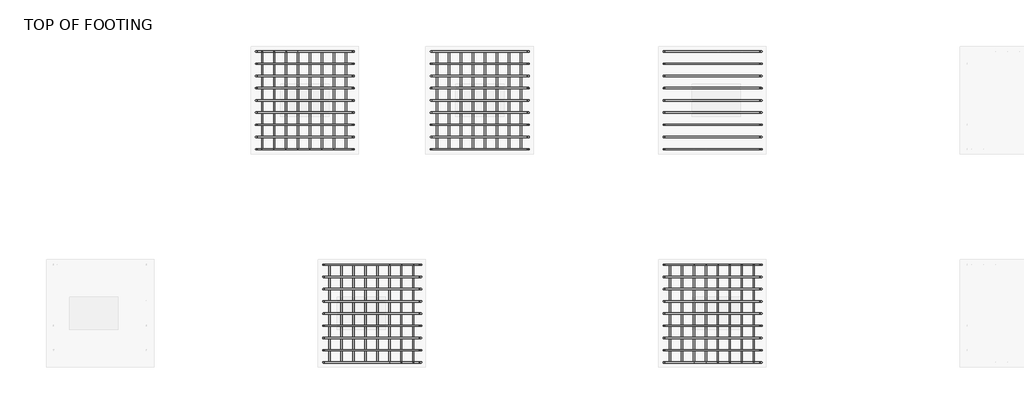
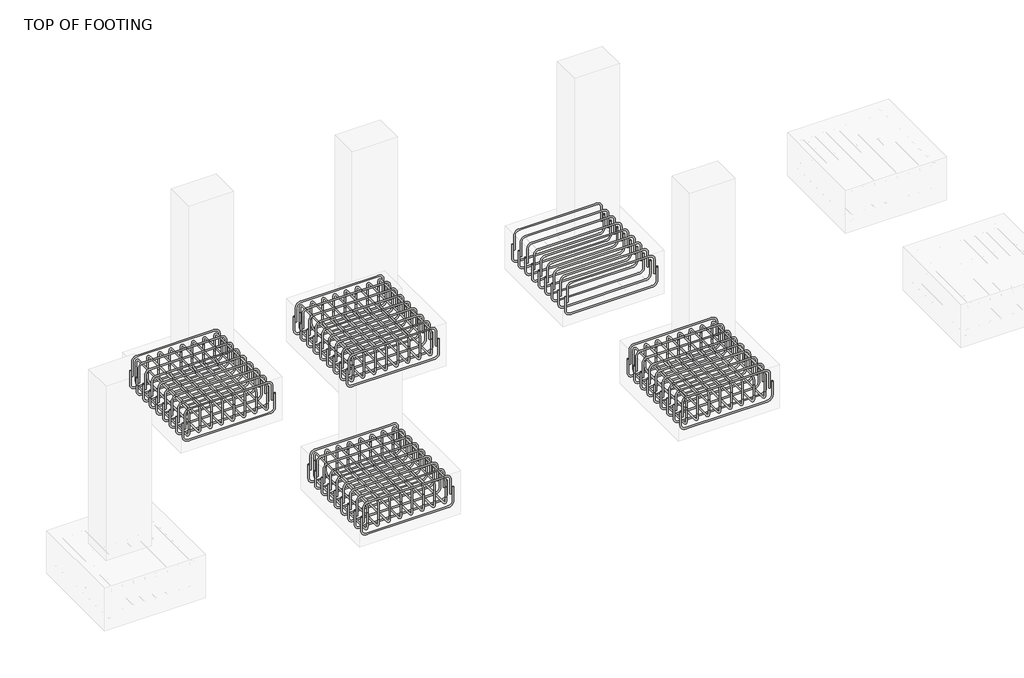
# One storey, part 17 of 20: 18 reinforcing bars.
"""IFC4 building model written with IfcOpenShell, lengths in millimetres."""

from ifc_helpers import new_model, si_unit, point, frame, origin, place, context, project, spatial, polyline, circle_curve, trimmed, segment, composite_curve, source, transform, mapped, element, save
from ifc_brep_helpers import swept_disk

model = new_model("IFC4")

# Units and contexts
model_context = context("Model", 3, world=origin())
ifc_project = project(units=[si_unit("LENGTHUNIT", "METRE", prefix="MILLI")], contexts=[model_context])

# Site, building, storey
site = spatial("IfcSite", under=ifc_project)
building = spatial("IfcBuilding", under=site)
storey = spatial("IfcBuildingStorey", under=building, Name="TOP OF FOOTING", Elevation=-1828.8)

# Reinforcing bars
placement = place(None, origin())
reinforcing_bar_shape = source(origin(), model_context, "Body", "SolidModel", [
    swept_disk(composite_curve([segment(polyline([(6636.1748054, 14441.1679708, -2006.6587682), (6636.1748054, 14441.1679708, -2153.9587682)]), True, "CONTINUOUS"), segment(trimmed(circle_curve(frame((6589.8248054, 14441.1679708, -2153.9587682), z_axis=(0.0, 1.0, 0.0), x_axis=(46.350000000000364, 0.0, 0.0)), 46.35), [point((6636.1748054, 14441.1679708, -2153.9587682))], [point((6589.8248054, 14441.1679708, -2200.3087682))], True, "CARTESIAN"), True, "CONTINUOUS"), segment(polyline([(6589.8248054, 14441.1679708, -2200.3087682), (5775.2248054, 14441.1679708, -2200.3087682)]), True, "CONTINUOUS"), segment(trimmed(circle_curve(frame((5775.2248054, 14441.1679708, -2153.9587682), z_axis=(0.0, 1.0, 0.0), x_axis=(0.0, 0.0, -46.34999999999991)), 46.35), [point((5775.2248054, 14441.1679708, -2200.3087682))], [point((5728.8748054, 14441.1679708, -2153.9587682))], True, "CARTESIAN"), True, "CONTINUOUS"), segment(polyline([(5728.8748054, 14441.1679708, -2153.9587682), (5728.8748054, 14441.1679708, -2006.6587682)]), True, "CONTINUOUS")], self_intersect=False), 6.35),
])
element("IfcReinforcingBar", 1, at=placement, inside=storey, context=model_context, shape_type="MappedRepresentation", body=[
    mapped(reinforcing_bar_shape, transform((0.0, 0.0, 0.0), x_axis=(1.0, 0.0, 0.0), y_axis=(0.0, 1.0, 0.0), z_axis=(0.0, 0.0, 1.0))),
    mapped(reinforcing_bar_shape, transform((0.0, -113.4125, 0.0), x_axis=(1.0, 0.0, 0.0), y_axis=(0.0, 1.0, 0.0), z_axis=(0.0, 0.0, 1.0))),
    mapped(reinforcing_bar_shape, transform((0.0, -226.825, 0.0), x_axis=(1.0, 0.0, 0.0), y_axis=(0.0, 1.0, 0.0), z_axis=(0.0, 0.0, 1.0))),
    mapped(reinforcing_bar_shape, transform((0.0, -340.2375, 0.0), x_axis=(1.0, 0.0, 0.0), y_axis=(0.0, 1.0, 0.0), z_axis=(0.0, 0.0, 1.0))),
    mapped(reinforcing_bar_shape, transform((0.0, -453.65, 0.0), x_axis=(1.0, 0.0, 0.0), y_axis=(0.0, 1.0, 0.0), z_axis=(0.0, 0.0, 1.0))),
    mapped(reinforcing_bar_shape, transform((0.0, -567.0625, 0.0), x_axis=(1.0, 0.0, 0.0), y_axis=(0.0, 1.0, 0.0), z_axis=(0.0, 0.0, 1.0))),
    mapped(reinforcing_bar_shape, transform((0.0, -680.475, 0.0), x_axis=(1.0, 0.0, 0.0), y_axis=(0.0, 1.0, 0.0), z_axis=(0.0, 0.0, 1.0))),
    mapped(reinforcing_bar_shape, transform((0.0, -793.8875, 0.0), x_axis=(1.0, 0.0, 0.0), y_axis=(0.0, 1.0, 0.0), z_axis=(0.0, 0.0, 1.0))),
    mapped(reinforcing_bar_shape, transform((0.0, -907.3, 0.0), x_axis=(1.0, 0.0, 0.0), y_axis=(0.0, 1.0, 0.0), z_axis=(0.0, 0.0, 1.0))),
])
reinforcing_bar_2_shape = source(origin(), model_context, "Body", "SolidModel", [
    swept_disk(composite_curve([segment(polyline([(5748.3489167, 14441.1679708, -2068.8), (5748.3489167, 14441.1679708, -1921.5)]), True, "CONTINUOUS"), segment(trimmed(circle_curve(frame((5794.6989167, 14441.1679708, -1921.5), z_axis=(0.0, 1.0, 0.0), x_axis=(-46.350000000000364, 0.0, 0.0)), 46.35), [point((5748.3489167, 14441.1679708, -1921.5))], [point((5794.6989167, 14441.1679708, -1875.15))], True, "CARTESIAN"), True, "CONTINUOUS"), segment(polyline([(5794.6989167, 14441.1679708, -1875.15), (6564.1623164, 14441.1679708, -1875.15)]), True, "CONTINUOUS"), segment(trimmed(circle_curve(frame((6564.1623164, 14441.1679708, -1921.5), z_axis=(0.0, 1.0, 0.0), x_axis=(0.0, 0.0, 46.34999999999991)), 46.35), [point((6564.1623164, 14441.1679708, -1875.15))], [point((6610.5123164, 14441.1679708, -1921.5))], True, "CARTESIAN"), True, "CONTINUOUS"), segment(polyline([(6610.5123164, 14441.1679708, -1921.5), (6610.5123164, 14441.1679708, -2068.8)]), True, "CONTINUOUS")], self_intersect=False), 6.35),
])
element("IfcReinforcingBar", 2, at=placement, inside=storey, context=model_context, shape_type="MappedRepresentation", body=[
    mapped(reinforcing_bar_2_shape, transform((0.0, 0.0, 0.0), x_axis=(1.0, 0.0, 0.0), y_axis=(0.0, 1.0, 0.0), z_axis=(0.0, 0.0, 1.0))),
    mapped(reinforcing_bar_2_shape, transform((0.0, -113.4125, 0.0), x_axis=(1.0, 0.0, 0.0), y_axis=(0.0, 1.0, 0.0), z_axis=(0.0, 0.0, 1.0))),
    mapped(reinforcing_bar_2_shape, transform((0.0, -226.825, 0.0), x_axis=(1.0, 0.0, 0.0), y_axis=(0.0, 1.0, 0.0), z_axis=(0.0, 0.0, 1.0))),
    mapped(reinforcing_bar_2_shape, transform((0.0, -340.2375, 0.0), x_axis=(1.0, 0.0, 0.0), y_axis=(0.0, 1.0, 0.0), z_axis=(0.0, 0.0, 1.0))),
    mapped(reinforcing_bar_2_shape, transform((0.0, -453.65, 0.0), x_axis=(1.0, 0.0, 0.0), y_axis=(0.0, 1.0, 0.0), z_axis=(0.0, 0.0, 1.0))),
    mapped(reinforcing_bar_2_shape, transform((0.0, -567.0625, 0.0), x_axis=(1.0, 0.0, 0.0), y_axis=(0.0, 1.0, 0.0), z_axis=(0.0, 0.0, 1.0))),
    mapped(reinforcing_bar_2_shape, transform((0.0, -680.475, 0.0), x_axis=(1.0, 0.0, 0.0), y_axis=(0.0, 1.0, 0.0), z_axis=(0.0, 0.0, 1.0))),
    mapped(reinforcing_bar_2_shape, transform((0.0, -793.8875, 0.0), x_axis=(1.0, 0.0, 0.0), y_axis=(0.0, 1.0, 0.0), z_axis=(0.0, 0.0, 1.0))),
    mapped(reinforcing_bar_2_shape, transform((0.0, -907.3, 0.0), x_axis=(1.0, 0.0, 0.0), y_axis=(0.0, 1.0, 0.0), z_axis=(0.0, 0.0, 1.0))),
])
reinforcing_bar_3_shape = source(origin(), model_context, "Body", "SolidModel", [
    swept_disk(composite_curve([segment(polyline([(6564.677844, 14441.1679708, -2086.1951968), (6564.677844, 14441.1679708, -1938.8951968)]), True, "CONTINUOUS"), segment(trimmed(circle_curve(frame((6564.677844, 14394.8179708, -1938.8951968), z_axis=(1.0, 0.0, 0.0), x_axis=(0.0, 46.349999999998545, 0.0)), 46.35), [point((6564.677844, 14441.1679708, -1938.8951968))], [point((6564.677844, 14394.8179708, -1892.5451968))], True, "CARTESIAN"), True, "CONTINUOUS"), segment(polyline([(6564.677844, 14394.8179708, -1892.5451968), (6564.677844, 13580.2179708, -1892.5451968)]), True, "CONTINUOUS"), segment(trimmed(circle_curve(frame((6564.677844, 13580.2179708, -1938.8951968), z_axis=(1.0, 0.0, 0.0), x_axis=(0.0, 0.0, 46.34999999999991)), 46.35), [point((6564.677844, 13580.2179708, -1892.5451968))], [point((6564.677844, 13533.8679708, -1938.8951968))], True, "CARTESIAN"), True, "CONTINUOUS"), segment(polyline([(6564.677844, 13533.8679708, -1938.8951968), (6564.677844, 13533.8679708, -2086.1951968)]), True, "CONTINUOUS")], self_intersect=False), 6.35),
])
element("IfcReinforcingBar", 3, at=placement, inside=storey, context=model_context, shape_type="MappedRepresentation", body=[
    mapped(reinforcing_bar_3_shape, transform((0.0, 0.0, 0.0), x_axis=(1.0, 0.0, 0.0), y_axis=(0.0, 1.0, 0.0), z_axis=(0.0, 0.0, 1.0))),
    mapped(reinforcing_bar_3_shape, transform((-111.2862402, 0.0, 0.0), x_axis=(1.0, 0.0, 0.0), y_axis=(0.0, 1.0, 0.0), z_axis=(0.0, 0.0, 1.0))),
    mapped(reinforcing_bar_3_shape, transform((-222.5724804, 0.0, 0.0), x_axis=(1.0, 0.0, 0.0), y_axis=(0.0, 1.0, 0.0), z_axis=(0.0, 0.0, 1.0))),
    mapped(reinforcing_bar_3_shape, transform((-333.8587205, 0.0, 0.0), x_axis=(1.0, 0.0, 0.0), y_axis=(0.0, 1.0, 0.0), z_axis=(0.0, 0.0, 1.0))),
    mapped(reinforcing_bar_3_shape, transform((-445.1449607, 0.0, 0.0), x_axis=(1.0, 0.0, 0.0), y_axis=(0.0, 1.0, 0.0), z_axis=(0.0, 0.0, 1.0))),
    mapped(reinforcing_bar_3_shape, transform((-556.4312009, 0.0, 0.0), x_axis=(1.0, 0.0, 0.0), y_axis=(0.0, 1.0, 0.0), z_axis=(0.0, 0.0, 1.0))),
    mapped(reinforcing_bar_3_shape, transform((-667.7174411, 0.0, 0.0), x_axis=(1.0, 0.0, 0.0), y_axis=(0.0, 1.0, 0.0), z_axis=(0.0, 0.0, 1.0))),
    mapped(reinforcing_bar_3_shape, transform((-779.0036813, 0.0, 0.0), x_axis=(1.0, 0.0, 0.0), y_axis=(0.0, 1.0, 0.0), z_axis=(0.0, 0.0, 1.0))),
])
reinforcing_bar_4_shape = source(origin(), model_context, "Body", "SolidModel", [
    swept_disk(composite_curve([segment(polyline([(5785.6741627, 14441.1679708, -1979.1645013), (5785.6741627, 14441.1679708, -2126.4645013)]), True, "CONTINUOUS"), segment(trimmed(circle_curve(frame((5785.6741627, 14394.8179708, -2126.4645013), z_axis=(-1.0, 0.0, 0.0), x_axis=(0.0, 46.349999999998545, 0.0)), 46.35), [point((5785.6741627, 14441.1679708, -2126.4645013))], [point((5785.6741627, 14394.8179708, -2172.8145013))], True, "CARTESIAN"), True, "CONTINUOUS"), segment(polyline([(5785.6741627, 14394.8179708, -2172.8145013), (5785.6741627, 13580.2179708, -2172.8145013)]), True, "CONTINUOUS"), segment(trimmed(circle_curve(frame((5785.6741627, 13580.2179708, -2126.4645013), z_axis=(-1.0, 0.0, 0.0), x_axis=(0.0, 0.0, -46.34999999999991)), 46.35), [point((5785.6741627, 13580.2179708, -2172.8145013))], [point((5785.6741627, 13533.8679708, -2126.4645013))], True, "CARTESIAN"), True, "CONTINUOUS"), segment(polyline([(5785.6741627, 13533.8679708, -2126.4645013), (5785.6741627, 13533.8679708, -1979.1645013)]), True, "CONTINUOUS")], self_intersect=False), 6.35),
])
element("IfcReinforcingBar", 4, at=placement, inside=storey, context=model_context, shape_type="MappedRepresentation", body=[
    mapped(reinforcing_bar_4_shape, transform((0.0, 0.0, 0.0), x_axis=(1.0, 0.0, 0.0), y_axis=(0.0, 1.0, 0.0), z_axis=(0.0, 0.0, 1.0))),
    mapped(reinforcing_bar_4_shape, transform((111.2862402, 0.0, 0.0), x_axis=(1.0, 0.0, 0.0), y_axis=(0.0, 1.0, 0.0), z_axis=(0.0, 0.0, 1.0))),
    mapped(reinforcing_bar_4_shape, transform((222.5724804, 0.0, 0.0), x_axis=(1.0, 0.0, 0.0), y_axis=(0.0, 1.0, 0.0), z_axis=(0.0, 0.0, 1.0))),
    mapped(reinforcing_bar_4_shape, transform((333.8587205, 0.0, 0.0), x_axis=(1.0, 0.0, 0.0), y_axis=(0.0, 1.0, 0.0), z_axis=(0.0, 0.0, 1.0))),
    mapped(reinforcing_bar_4_shape, transform((445.1449607, 0.0, 0.0), x_axis=(1.0, 0.0, 0.0), y_axis=(0.0, 1.0, 0.0), z_axis=(0.0, 0.0, 1.0))),
    mapped(reinforcing_bar_4_shape, transform((556.4312009, 0.0, 0.0), x_axis=(1.0, 0.0, 0.0), y_axis=(0.0, 1.0, 0.0), z_axis=(0.0, 0.0, 1.0))),
    mapped(reinforcing_bar_4_shape, transform((667.7174411, 0.0, 0.0), x_axis=(1.0, 0.0, 0.0), y_axis=(0.0, 1.0, 0.0), z_axis=(0.0, 0.0, 1.0))),
    mapped(reinforcing_bar_4_shape, transform((779.0036813, 0.0, 0.0), x_axis=(1.0, 0.0, 0.0), y_axis=(0.0, 1.0, 0.0), z_axis=(0.0, 0.0, 1.0))),
])
reinforcing_bar_5_shape = source(origin(), model_context, "Body", "SolidModel", [
    swept_disk(composite_curve([segment(polyline([(8260.5179014, 14441.1679708, -2006.6587682), (8260.5179014, 14441.1679708, -2153.9587682)]), True, "CONTINUOUS"), segment(trimmed(circle_curve(frame((8214.1679014, 14441.1679708, -2153.9587682), z_axis=(0.0, 1.0, 0.0), x_axis=(46.350000000000364, 0.0, 0.0)), 46.35), [point((8260.5179014, 14441.1679708, -2153.9587682))], [point((8214.1679014, 14441.1679708, -2200.3087682))], True, "CARTESIAN"), True, "CONTINUOUS"), segment(polyline([(8214.1679014, 14441.1679708, -2200.3087682), (7399.5679014, 14441.1679708, -2200.3087682)]), True, "CONTINUOUS"), segment(trimmed(circle_curve(frame((7399.5679014, 14441.1679708, -2153.9587682), z_axis=(0.0, 1.0, 0.0), x_axis=(0.0, 0.0, -46.34999999999991)), 46.35), [point((7399.5679014, 14441.1679708, -2200.3087682))], [point((7353.2179014, 14441.1679708, -2153.9587682))], True, "CARTESIAN"), True, "CONTINUOUS"), segment(polyline([(7353.2179014, 14441.1679708, -2153.9587682), (7353.2179014, 14441.1679708, -2006.6587682)]), True, "CONTINUOUS")], self_intersect=False), 6.35),
])
element("IfcReinforcingBar", 5, at=placement, inside=storey, context=model_context, shape_type="MappedRepresentation", body=[
    mapped(reinforcing_bar_5_shape, transform((0.0, 0.0, 0.0), x_axis=(1.0, 0.0, 0.0), y_axis=(0.0, 1.0, 0.0), z_axis=(0.0, 0.0, 1.0))),
    mapped(reinforcing_bar_5_shape, transform((0.0, -113.4125, 0.0), x_axis=(1.0, 0.0, 0.0), y_axis=(0.0, 1.0, 0.0), z_axis=(0.0, 0.0, 1.0))),
    mapped(reinforcing_bar_5_shape, transform((0.0, -226.825, 0.0), x_axis=(1.0, 0.0, 0.0), y_axis=(0.0, 1.0, 0.0), z_axis=(0.0, 0.0, 1.0))),
    mapped(reinforcing_bar_5_shape, transform((0.0, -340.2375, 0.0), x_axis=(1.0, 0.0, 0.0), y_axis=(0.0, 1.0, 0.0), z_axis=(0.0, 0.0, 1.0))),
    mapped(reinforcing_bar_5_shape, transform((0.0, -453.65, 0.0), x_axis=(1.0, 0.0, 0.0), y_axis=(0.0, 1.0, 0.0), z_axis=(0.0, 0.0, 1.0))),
    mapped(reinforcing_bar_5_shape, transform((0.0, -567.0625, 0.0), x_axis=(1.0, 0.0, 0.0), y_axis=(0.0, 1.0, 0.0), z_axis=(0.0, 0.0, 1.0))),
    mapped(reinforcing_bar_5_shape, transform((0.0, -680.475, 0.0), x_axis=(1.0, 0.0, 0.0), y_axis=(0.0, 1.0, 0.0), z_axis=(0.0, 0.0, 1.0))),
    mapped(reinforcing_bar_5_shape, transform((0.0, -793.8875, 0.0), x_axis=(1.0, 0.0, 0.0), y_axis=(0.0, 1.0, 0.0), z_axis=(0.0, 0.0, 1.0))),
    mapped(reinforcing_bar_5_shape, transform((0.0, -907.3, 0.0), x_axis=(1.0, 0.0, 0.0), y_axis=(0.0, 1.0, 0.0), z_axis=(0.0, 0.0, 1.0))),
])
reinforcing_bar_6_shape = source(origin(), model_context, "Body", "SolidModel", [
    swept_disk(composite_curve([segment(polyline([(7372.6920127, 14441.1679708, -2068.8), (7372.6920127, 14441.1679708, -1921.5)]), True, "CONTINUOUS"), segment(trimmed(circle_curve(frame((7419.0420127, 14441.1679708, -1921.5), z_axis=(0.0, 1.0, 0.0), x_axis=(-46.349999999999454, 0.0, 0.0)), 46.35), [point((7372.6920127, 14441.1679708, -1921.5))], [point((7419.0420127, 14441.1679708, -1875.15))], True, "CARTESIAN"), True, "CONTINUOUS"), segment(polyline([(7419.0420127, 14441.1679708, -1875.15), (8188.5054124, 14441.1679708, -1875.15)]), True, "CONTINUOUS"), segment(trimmed(circle_curve(frame((8188.5054124, 14441.1679708, -1921.5), z_axis=(0.0, 1.0, 0.0), x_axis=(0.0, 0.0, 46.34999999999991)), 46.35), [point((8188.5054124, 14441.1679708, -1875.15))], [point((8234.8554124, 14441.1679708, -1921.5))], True, "CARTESIAN"), True, "CONTINUOUS"), segment(polyline([(8234.8554124, 14441.1679708, -1921.5), (8234.8554124, 14441.1679708, -2068.8)]), True, "CONTINUOUS")], self_intersect=False), 6.35),
])
element("IfcReinforcingBar", 6, at=placement, inside=storey, context=model_context, shape_type="MappedRepresentation", body=[
    mapped(reinforcing_bar_6_shape, transform((0.0, 0.0, 0.0), x_axis=(1.0, 0.0, 0.0), y_axis=(0.0, 1.0, 0.0), z_axis=(0.0, 0.0, 1.0))),
    mapped(reinforcing_bar_6_shape, transform((0.0, -113.4125, 0.0), x_axis=(1.0, 0.0, 0.0), y_axis=(0.0, 1.0, 0.0), z_axis=(0.0, 0.0, 1.0))),
    mapped(reinforcing_bar_6_shape, transform((0.0, -226.825, 0.0), x_axis=(1.0, 0.0, 0.0), y_axis=(0.0, 1.0, 0.0), z_axis=(0.0, 0.0, 1.0))),
    mapped(reinforcing_bar_6_shape, transform((0.0, -340.2375, 0.0), x_axis=(1.0, 0.0, 0.0), y_axis=(0.0, 1.0, 0.0), z_axis=(0.0, 0.0, 1.0))),
    mapped(reinforcing_bar_6_shape, transform((0.0, -453.65, 0.0), x_axis=(1.0, 0.0, 0.0), y_axis=(0.0, 1.0, 0.0), z_axis=(0.0, 0.0, 1.0))),
    mapped(reinforcing_bar_6_shape, transform((0.0, -567.0625, 0.0), x_axis=(1.0, 0.0, 0.0), y_axis=(0.0, 1.0, 0.0), z_axis=(0.0, 0.0, 1.0))),
    mapped(reinforcing_bar_6_shape, transform((0.0, -680.475, 0.0), x_axis=(1.0, 0.0, 0.0), y_axis=(0.0, 1.0, 0.0), z_axis=(0.0, 0.0, 1.0))),
    mapped(reinforcing_bar_6_shape, transform((0.0, -793.8875, 0.0), x_axis=(1.0, 0.0, 0.0), y_axis=(0.0, 1.0, 0.0), z_axis=(0.0, 0.0, 1.0))),
    mapped(reinforcing_bar_6_shape, transform((0.0, -907.3, 0.0), x_axis=(1.0, 0.0, 0.0), y_axis=(0.0, 1.0, 0.0), z_axis=(0.0, 0.0, 1.0))),
])
reinforcing_bar_7_shape = source(origin(), model_context, "Body", "SolidModel", [
    swept_disk(composite_curve([segment(polyline([(8189.02094, 14441.1679708, -2086.1951968), (8189.02094, 14441.1679708, -1938.8951968)]), True, "CONTINUOUS"), segment(trimmed(circle_curve(frame((8189.02094, 14394.8179708, -1938.8951968), z_axis=(1.0, 0.0, 0.0), x_axis=(0.0, 46.349999999998545, 0.0)), 46.35), [point((8189.02094, 14441.1679708, -1938.8951968))], [point((8189.02094, 14394.8179708, -1892.5451968))], True, "CARTESIAN"), True, "CONTINUOUS"), segment(polyline([(8189.02094, 14394.8179708, -1892.5451968), (8189.02094, 13580.2179708, -1892.5451968)]), True, "CONTINUOUS"), segment(trimmed(circle_curve(frame((8189.02094, 13580.2179708, -1938.8951968), z_axis=(1.0, 0.0, 0.0), x_axis=(0.0, 0.0, 46.34999999999991)), 46.35), [point((8189.02094, 13580.2179708, -1892.5451968))], [point((8189.02094, 13533.8679708, -1938.8951968))], True, "CARTESIAN"), True, "CONTINUOUS"), segment(polyline([(8189.02094, 13533.8679708, -1938.8951968), (8189.02094, 13533.8679708, -2086.1951968)]), True, "CONTINUOUS")], self_intersect=False), 6.35),
])
element("IfcReinforcingBar", 7, at=placement, inside=storey, context=model_context, shape_type="MappedRepresentation", body=[
    mapped(reinforcing_bar_7_shape, transform((0.0, 0.0, 0.0), x_axis=(1.0, 0.0, 0.0), y_axis=(0.0, 1.0, 0.0), z_axis=(0.0, 0.0, 1.0))),
    mapped(reinforcing_bar_7_shape, transform((-111.2862402, 0.0, 0.0), x_axis=(1.0, 0.0, 0.0), y_axis=(0.0, 1.0, 0.0), z_axis=(0.0, 0.0, 1.0))),
    mapped(reinforcing_bar_7_shape, transform((-222.5724804, 0.0, 0.0), x_axis=(1.0, 0.0, 0.0), y_axis=(0.0, 1.0, 0.0), z_axis=(0.0, 0.0, 1.0))),
    mapped(reinforcing_bar_7_shape, transform((-333.8587205, 0.0, 0.0), x_axis=(1.0, 0.0, 0.0), y_axis=(0.0, 1.0, 0.0), z_axis=(0.0, 0.0, 1.0))),
    mapped(reinforcing_bar_7_shape, transform((-445.1449607, 0.0, 0.0), x_axis=(1.0, 0.0, 0.0), y_axis=(0.0, 1.0, 0.0), z_axis=(0.0, 0.0, 1.0))),
    mapped(reinforcing_bar_7_shape, transform((-556.4312009, 0.0, 0.0), x_axis=(1.0, 0.0, 0.0), y_axis=(0.0, 1.0, 0.0), z_axis=(0.0, 0.0, 1.0))),
    mapped(reinforcing_bar_7_shape, transform((-667.7174411, 0.0, 0.0), x_axis=(1.0, 0.0, 0.0), y_axis=(0.0, 1.0, 0.0), z_axis=(0.0, 0.0, 1.0))),
    mapped(reinforcing_bar_7_shape, transform((-779.0036813, 0.0, 0.0), x_axis=(1.0, 0.0, 0.0), y_axis=(0.0, 1.0, 0.0), z_axis=(0.0, 0.0, 1.0))),
])
reinforcing_bar_8_shape = source(origin(), model_context, "Body", "SolidModel", [
    swept_disk(composite_curve([segment(polyline([(7410.0172587, 14441.1679708, -1979.1645013), (7410.0172587, 14441.1679708, -2126.4645013)]), True, "CONTINUOUS"), segment(trimmed(circle_curve(frame((7410.0172587, 14394.8179708, -2126.4645013), z_axis=(-1.0, 0.0, 0.0), x_axis=(0.0, 46.349999999998545, 0.0)), 46.35), [point((7410.0172587, 14441.1679708, -2126.4645013))], [point((7410.0172587, 14394.8179708, -2172.8145013))], True, "CARTESIAN"), True, "CONTINUOUS"), segment(polyline([(7410.0172587, 14394.8179708, -2172.8145013), (7410.0172587, 13580.2179708, -2172.8145013)]), True, "CONTINUOUS"), segment(trimmed(circle_curve(frame((7410.0172587, 13580.2179708, -2126.4645013), z_axis=(-1.0, 0.0, 0.0), x_axis=(0.0, 0.0, -46.34999999999991)), 46.35), [point((7410.0172587, 13580.2179708, -2172.8145013))], [point((7410.0172587, 13533.8679708, -2126.4645013))], True, "CARTESIAN"), True, "CONTINUOUS"), segment(polyline([(7410.0172587, 13533.8679708, -2126.4645013), (7410.0172587, 13533.8679708, -1979.1645013)]), True, "CONTINUOUS")], self_intersect=False), 6.35),
])
element("IfcReinforcingBar", 8, at=placement, inside=storey, context=model_context, shape_type="MappedRepresentation", body=[
    mapped(reinforcing_bar_8_shape, transform((0.0, 0.0, 0.0), x_axis=(1.0, 0.0, 0.0), y_axis=(0.0, 1.0, 0.0), z_axis=(0.0, 0.0, 1.0))),
    mapped(reinforcing_bar_8_shape, transform((111.2862402, 0.0, 0.0), x_axis=(1.0, 0.0, 0.0), y_axis=(0.0, 1.0, 0.0), z_axis=(0.0, 0.0, 1.0))),
    mapped(reinforcing_bar_8_shape, transform((222.5724804, 0.0, 0.0), x_axis=(1.0, 0.0, 0.0), y_axis=(0.0, 1.0, 0.0), z_axis=(0.0, 0.0, 1.0))),
    mapped(reinforcing_bar_8_shape, transform((333.8587205, 0.0, 0.0), x_axis=(1.0, 0.0, 0.0), y_axis=(0.0, 1.0, 0.0), z_axis=(0.0, 0.0, 1.0))),
    mapped(reinforcing_bar_8_shape, transform((445.1449607, 0.0, 0.0), x_axis=(1.0, 0.0, 0.0), y_axis=(0.0, 1.0, 0.0), z_axis=(0.0, 0.0, 1.0))),
    mapped(reinforcing_bar_8_shape, transform((556.4312009, 0.0, 0.0), x_axis=(1.0, 0.0, 0.0), y_axis=(0.0, 1.0, 0.0), z_axis=(0.0, 0.0, 1.0))),
    mapped(reinforcing_bar_8_shape, transform((667.7174411, 0.0, 0.0), x_axis=(1.0, 0.0, 0.0), y_axis=(0.0, 1.0, 0.0), z_axis=(0.0, 0.0, 1.0))),
    mapped(reinforcing_bar_8_shape, transform((779.0036813, 0.0, 0.0), x_axis=(1.0, 0.0, 0.0), y_axis=(0.0, 1.0, 0.0), z_axis=(0.0, 0.0, 1.0))),
])
reinforcing_bar_9_shape = source(origin(), model_context, "Body", "SolidModel", [
    swept_disk(composite_curve([segment(polyline([(10422.7663908, 14441.1679708, -2006.6587682), (10422.7663908, 14441.1679708, -2153.9587682)]), True, "CONTINUOUS"), segment(trimmed(circle_curve(frame((10376.4163908, 14441.1679708, -2153.9587682), z_axis=(0.0, 1.0, 0.0), x_axis=(46.350000000000364, 0.0, 0.0)), 46.35), [point((10422.7663908, 14441.1679708, -2153.9587682))], [point((10376.4163908, 14441.1679708, -2200.3087682))], True, "CARTESIAN"), True, "CONTINUOUS"), segment(polyline([(10376.4163908, 14441.1679708, -2200.3087682), (9561.8163908, 14441.1679708, -2200.3087682)]), True, "CONTINUOUS"), segment(trimmed(circle_curve(frame((9561.8163908, 14441.1679708, -2153.9587682), z_axis=(0.0, 1.0, 0.0), x_axis=(0.0, 0.0, -46.34999999999991)), 46.35), [point((9561.8163908, 14441.1679708, -2200.3087682))], [point((9515.4663908, 14441.1679708, -2153.9587682))], True, "CARTESIAN"), True, "CONTINUOUS"), segment(polyline([(9515.4663908, 14441.1679708, -2153.9587682), (9515.4663908, 14441.1679708, -2006.6587682)]), True, "CONTINUOUS")], self_intersect=False), 6.35),
])
element("IfcReinforcingBar", 9, at=placement, inside=storey, context=model_context, shape_type="MappedRepresentation", body=[
    mapped(reinforcing_bar_9_shape, transform((0.0, 0.0, 0.0), x_axis=(1.0, 0.0, 0.0), y_axis=(0.0, 1.0, 0.0), z_axis=(0.0, 0.0, 1.0))),
    mapped(reinforcing_bar_9_shape, transform((0.0, -113.4125, 0.0), x_axis=(1.0, 0.0, 0.0), y_axis=(0.0, 1.0, 0.0), z_axis=(0.0, 0.0, 1.0))),
    mapped(reinforcing_bar_9_shape, transform((0.0, -226.825, 0.0), x_axis=(1.0, 0.0, 0.0), y_axis=(0.0, 1.0, 0.0), z_axis=(0.0, 0.0, 1.0))),
    mapped(reinforcing_bar_9_shape, transform((0.0, -340.2375, 0.0), x_axis=(1.0, 0.0, 0.0), y_axis=(0.0, 1.0, 0.0), z_axis=(0.0, 0.0, 1.0))),
    mapped(reinforcing_bar_9_shape, transform((0.0, -453.65, 0.0), x_axis=(1.0, 0.0, 0.0), y_axis=(0.0, 1.0, 0.0), z_axis=(0.0, 0.0, 1.0))),
    mapped(reinforcing_bar_9_shape, transform((0.0, -567.0625, 0.0), x_axis=(1.0, 0.0, 0.0), y_axis=(0.0, 1.0, 0.0), z_axis=(0.0, 0.0, 1.0))),
    mapped(reinforcing_bar_9_shape, transform((0.0, -680.475, 0.0), x_axis=(1.0, 0.0, 0.0), y_axis=(0.0, 1.0, 0.0), z_axis=(0.0, 0.0, 1.0))),
    mapped(reinforcing_bar_9_shape, transform((0.0, -793.8875, 0.0), x_axis=(1.0, 0.0, 0.0), y_axis=(0.0, 1.0, 0.0), z_axis=(0.0, 0.0, 1.0))),
    mapped(reinforcing_bar_9_shape, transform((0.0, -907.3, 0.0), x_axis=(1.0, 0.0, 0.0), y_axis=(0.0, 1.0, 0.0), z_axis=(0.0, 0.0, 1.0))),
])
reinforcing_bar_10_shape = source(origin(), model_context, "Body", "SolidModel", [
    swept_disk(composite_curve([segment(polyline([(9534.9405021, 14441.1679708, -2068.8), (9534.9405021, 14441.1679708, -1921.5)]), True, "CONTINUOUS"), segment(trimmed(circle_curve(frame((9581.2905021, 14441.1679708, -1921.5), z_axis=(0.0, 1.0, 0.0), x_axis=(-46.350000000000364, 0.0, 0.0)), 46.35), [point((9534.9405021, 14441.1679708, -1921.5))], [point((9581.2905021, 14441.1679708, -1875.15))], True, "CARTESIAN"), True, "CONTINUOUS"), segment(polyline([(9581.2905021, 14441.1679708, -1875.15), (10350.7539017, 14441.1679708, -1875.15)]), True, "CONTINUOUS"), segment(trimmed(circle_curve(frame((10350.7539017, 14441.1679708, -1921.5), z_axis=(0.0, 1.0, 0.0), x_axis=(0.0, 0.0, 46.34999999999991)), 46.35), [point((10350.7539017, 14441.1679708, -1875.15))], [point((10397.1039017, 14441.1679708, -1921.5))], True, "CARTESIAN"), True, "CONTINUOUS"), segment(polyline([(10397.1039017, 14441.1679708, -1921.5), (10397.1039017, 14441.1679708, -2068.8)]), True, "CONTINUOUS")], self_intersect=False), 6.35),
])
element("IfcReinforcingBar", 10, at=placement, inside=storey, context=model_context, shape_type="MappedRepresentation", body=[
    mapped(reinforcing_bar_10_shape, transform((0.0, 0.0, 0.0), x_axis=(1.0, 0.0, 0.0), y_axis=(0.0, 1.0, 0.0), z_axis=(0.0, 0.0, 1.0))),
    mapped(reinforcing_bar_10_shape, transform((0.0, -113.4125, 0.0), x_axis=(1.0, 0.0, 0.0), y_axis=(0.0, 1.0, 0.0), z_axis=(0.0, 0.0, 1.0))),
    mapped(reinforcing_bar_10_shape, transform((0.0, -226.825, 0.0), x_axis=(1.0, 0.0, 0.0), y_axis=(0.0, 1.0, 0.0), z_axis=(0.0, 0.0, 1.0))),
    mapped(reinforcing_bar_10_shape, transform((0.0, -340.2375, 0.0), x_axis=(1.0, 0.0, 0.0), y_axis=(0.0, 1.0, 0.0), z_axis=(0.0, 0.0, 1.0))),
    mapped(reinforcing_bar_10_shape, transform((0.0, -453.65, 0.0), x_axis=(1.0, 0.0, 0.0), y_axis=(0.0, 1.0, 0.0), z_axis=(0.0, 0.0, 1.0))),
    mapped(reinforcing_bar_10_shape, transform((0.0, -567.0625, 0.0), x_axis=(1.0, 0.0, 0.0), y_axis=(0.0, 1.0, 0.0), z_axis=(0.0, 0.0, 1.0))),
    mapped(reinforcing_bar_10_shape, transform((0.0, -680.475, 0.0), x_axis=(1.0, 0.0, 0.0), y_axis=(0.0, 1.0, 0.0), z_axis=(0.0, 0.0, 1.0))),
    mapped(reinforcing_bar_10_shape, transform((0.0, -793.8875, 0.0), x_axis=(1.0, 0.0, 0.0), y_axis=(0.0, 1.0, 0.0), z_axis=(0.0, 0.0, 1.0))),
    mapped(reinforcing_bar_10_shape, transform((0.0, -907.3, 0.0), x_axis=(1.0, 0.0, 0.0), y_axis=(0.0, 1.0, 0.0), z_axis=(0.0, 0.0, 1.0))),
])
reinforcing_bar_11_shape = source(origin(), model_context, "Body", "SolidModel", [
    swept_disk(composite_curve([segment(polyline([(10422.7663908, 12461.0575451, -2006.6587682), (10422.7663908, 12461.0575451, -2153.9587682)]), True, "CONTINUOUS"), segment(trimmed(circle_curve(frame((10376.4163908, 12461.0575451, -2153.9587682), z_axis=(0.0, 1.0, 0.0), x_axis=(46.350000000000364, 0.0, 0.0)), 46.35), [point((10422.7663908, 12461.0575451, -2153.9587682))], [point((10376.4163908, 12461.0575451, -2200.3087682))], True, "CARTESIAN"), True, "CONTINUOUS"), segment(polyline([(10376.4163908, 12461.0575451, -2200.3087682), (9561.8163908, 12461.0575451, -2200.3087682)]), True, "CONTINUOUS"), segment(trimmed(circle_curve(frame((9561.8163908, 12461.0575451, -2153.9587682), z_axis=(0.0, 1.0, 0.0), x_axis=(0.0, 0.0, -46.34999999999991)), 46.35), [point((9561.8163908, 12461.0575451, -2200.3087682))], [point((9515.4663908, 12461.0575451, -2153.9587682))], True, "CARTESIAN"), True, "CONTINUOUS"), segment(polyline([(9515.4663908, 12461.0575451, -2153.9587682), (9515.4663908, 12461.0575451, -2006.6587682)]), True, "CONTINUOUS")], self_intersect=False), 6.35),
])
element("IfcReinforcingBar", 11, at=placement, inside=storey, context=model_context, shape_type="MappedRepresentation", body=[
    mapped(reinforcing_bar_11_shape, transform((0.0, 0.0, 0.0), x_axis=(1.0, 0.0, 0.0), y_axis=(0.0, 1.0, 0.0), z_axis=(0.0, 0.0, 1.0))),
    mapped(reinforcing_bar_11_shape, transform((0.0, -113.4125, 0.0), x_axis=(1.0, 0.0, 0.0), y_axis=(0.0, 1.0, 0.0), z_axis=(0.0, 0.0, 1.0))),
    mapped(reinforcing_bar_11_shape, transform((0.0, -226.825, 0.0), x_axis=(1.0, 0.0, 0.0), y_axis=(0.0, 1.0, 0.0), z_axis=(0.0, 0.0, 1.0))),
    mapped(reinforcing_bar_11_shape, transform((0.0, -340.2375, 0.0), x_axis=(1.0, 0.0, 0.0), y_axis=(0.0, 1.0, 0.0), z_axis=(0.0, 0.0, 1.0))),
    mapped(reinforcing_bar_11_shape, transform((0.0, -453.65, 0.0), x_axis=(1.0, 0.0, 0.0), y_axis=(0.0, 1.0, 0.0), z_axis=(0.0, 0.0, 1.0))),
    mapped(reinforcing_bar_11_shape, transform((0.0, -567.0625, 0.0), x_axis=(1.0, 0.0, 0.0), y_axis=(0.0, 1.0, 0.0), z_axis=(0.0, 0.0, 1.0))),
    mapped(reinforcing_bar_11_shape, transform((0.0, -680.475, 0.0), x_axis=(1.0, 0.0, 0.0), y_axis=(0.0, 1.0, 0.0), z_axis=(0.0, 0.0, 1.0))),
    mapped(reinforcing_bar_11_shape, transform((0.0, -793.8875, 0.0), x_axis=(1.0, 0.0, 0.0), y_axis=(0.0, 1.0, 0.0), z_axis=(0.0, 0.0, 1.0))),
    mapped(reinforcing_bar_11_shape, transform((0.0, -907.3, 0.0), x_axis=(1.0, 0.0, 0.0), y_axis=(0.0, 1.0, 0.0), z_axis=(0.0, 0.0, 1.0))),
])
reinforcing_bar_12_shape = source(origin(), model_context, "Body", "SolidModel", [
    swept_disk(composite_curve([segment(polyline([(9534.9405021, 12461.0575451, -2068.8), (9534.9405021, 12461.0575451, -1921.5)]), True, "CONTINUOUS"), segment(trimmed(circle_curve(frame((9581.2905021, 12461.0575451, -1921.5), z_axis=(0.0, 1.0, 0.0), x_axis=(-46.350000000000364, 0.0, 0.0)), 46.35), [point((9534.9405021, 12461.0575451, -1921.5))], [point((9581.2905021, 12461.0575451, -1875.15))], True, "CARTESIAN"), True, "CONTINUOUS"), segment(polyline([(9581.2905021, 12461.0575451, -1875.15), (10350.7539017, 12461.0575451, -1875.15)]), True, "CONTINUOUS"), segment(trimmed(circle_curve(frame((10350.7539017, 12461.0575451, -1921.5), z_axis=(0.0, 1.0, 0.0), x_axis=(0.0, 0.0, 46.34999999999991)), 46.35), [point((10350.7539017, 12461.0575451, -1875.15))], [point((10397.1039017, 12461.0575451, -1921.5))], True, "CARTESIAN"), True, "CONTINUOUS"), segment(polyline([(10397.1039017, 12461.0575451, -1921.5), (10397.1039017, 12461.0575451, -2068.8)]), True, "CONTINUOUS")], self_intersect=False), 6.35),
])
element("IfcReinforcingBar", 12, at=placement, inside=storey, context=model_context, shape_type="MappedRepresentation", body=[
    mapped(reinforcing_bar_12_shape, transform((0.0, 0.0, 0.0), x_axis=(1.0, 0.0, 0.0), y_axis=(0.0, 1.0, 0.0), z_axis=(0.0, 0.0, 1.0))),
    mapped(reinforcing_bar_12_shape, transform((0.0, -113.4125, 0.0), x_axis=(1.0, 0.0, 0.0), y_axis=(0.0, 1.0, 0.0), z_axis=(0.0, 0.0, 1.0))),
    mapped(reinforcing_bar_12_shape, transform((0.0, -226.825, 0.0), x_axis=(1.0, 0.0, 0.0), y_axis=(0.0, 1.0, 0.0), z_axis=(0.0, 0.0, 1.0))),
    mapped(reinforcing_bar_12_shape, transform((0.0, -340.2375, 0.0), x_axis=(1.0, 0.0, 0.0), y_axis=(0.0, 1.0, 0.0), z_axis=(0.0, 0.0, 1.0))),
    mapped(reinforcing_bar_12_shape, transform((0.0, -453.65, 0.0), x_axis=(1.0, 0.0, 0.0), y_axis=(0.0, 1.0, 0.0), z_axis=(0.0, 0.0, 1.0))),
    mapped(reinforcing_bar_12_shape, transform((0.0, -567.0625, 0.0), x_axis=(1.0, 0.0, 0.0), y_axis=(0.0, 1.0, 0.0), z_axis=(0.0, 0.0, 1.0))),
    mapped(reinforcing_bar_12_shape, transform((0.0, -680.475, 0.0), x_axis=(1.0, 0.0, 0.0), y_axis=(0.0, 1.0, 0.0), z_axis=(0.0, 0.0, 1.0))),
    mapped(reinforcing_bar_12_shape, transform((0.0, -793.8875, 0.0), x_axis=(1.0, 0.0, 0.0), y_axis=(0.0, 1.0, 0.0), z_axis=(0.0, 0.0, 1.0))),
    mapped(reinforcing_bar_12_shape, transform((0.0, -907.3, 0.0), x_axis=(1.0, 0.0, 0.0), y_axis=(0.0, 1.0, 0.0), z_axis=(0.0, 0.0, 1.0))),
])
reinforcing_bar_13_shape = source(origin(), model_context, "Body", "SolidModel", [
    swept_disk(composite_curve([segment(polyline([(10351.2694294, 12461.0575451, -2086.1951968), (10351.2694294, 12461.0575451, -1938.8951968)]), True, "CONTINUOUS"), segment(trimmed(circle_curve(frame((10351.2694294, 12414.7075451, -1938.8951968), z_axis=(1.0, 0.0, 0.0), x_axis=(0.0, 46.350000000000364, 0.0)), 46.35), [point((10351.2694294, 12461.0575451, -1938.8951968))], [point((10351.2694294, 12414.7075451, -1892.5451968))], True, "CARTESIAN"), True, "CONTINUOUS"), segment(polyline([(10351.2694294, 12414.7075451, -1892.5451968), (10351.2694294, 11600.1075451, -1892.5451968)]), True, "CONTINUOUS"), segment(trimmed(circle_curve(frame((10351.2694294, 11600.1075451, -1938.8951968), z_axis=(1.0, 0.0, 0.0), x_axis=(0.0, 0.0, 46.34999999999991)), 46.35), [point((10351.2694294, 11600.1075451, -1892.5451968))], [point((10351.2694294, 11553.7575451, -1938.8951968))], True, "CARTESIAN"), True, "CONTINUOUS"), segment(polyline([(10351.2694294, 11553.7575451, -1938.8951968), (10351.2694294, 11553.7575451, -2086.1951968)]), True, "CONTINUOUS")], self_intersect=False), 6.35),
])
element("IfcReinforcingBar", 13, at=placement, inside=storey, context=model_context, shape_type="MappedRepresentation", body=[
    mapped(reinforcing_bar_13_shape, transform((0.0, 0.0, 0.0), x_axis=(1.0, 0.0, 0.0), y_axis=(0.0, 1.0, 0.0), z_axis=(0.0, 0.0, 1.0))),
    mapped(reinforcing_bar_13_shape, transform((-111.2862402, 0.0, 0.0), x_axis=(1.0, 0.0, 0.0), y_axis=(0.0, 1.0, 0.0), z_axis=(0.0, 0.0, 1.0))),
    mapped(reinforcing_bar_13_shape, transform((-222.5724804, 0.0, 0.0), x_axis=(1.0, 0.0, 0.0), y_axis=(0.0, 1.0, 0.0), z_axis=(0.0, 0.0, 1.0))),
    mapped(reinforcing_bar_13_shape, transform((-333.8587205, 0.0, 0.0), x_axis=(1.0, 0.0, 0.0), y_axis=(0.0, 1.0, 0.0), z_axis=(0.0, 0.0, 1.0))),
    mapped(reinforcing_bar_13_shape, transform((-445.1449607, 0.0, 0.0), x_axis=(1.0, 0.0, 0.0), y_axis=(0.0, 1.0, 0.0), z_axis=(0.0, 0.0, 1.0))),
    mapped(reinforcing_bar_13_shape, transform((-556.4312009, 0.0, 0.0), x_axis=(1.0, 0.0, 0.0), y_axis=(0.0, 1.0, 0.0), z_axis=(0.0, 0.0, 1.0))),
    mapped(reinforcing_bar_13_shape, transform((-667.7174411, 0.0, 0.0), x_axis=(1.0, 0.0, 0.0), y_axis=(0.0, 1.0, 0.0), z_axis=(0.0, 0.0, 1.0))),
    mapped(reinforcing_bar_13_shape, transform((-779.0036813, 0.0, 0.0), x_axis=(1.0, 0.0, 0.0), y_axis=(0.0, 1.0, 0.0), z_axis=(0.0, 0.0, 1.0))),
])
reinforcing_bar_14_shape = source(origin(), model_context, "Body", "SolidModel", [
    swept_disk(composite_curve([segment(polyline([(9572.2657481, 12461.0575451, -1979.1645013), (9572.2657481, 12461.0575451, -2126.4645013)]), True, "CONTINUOUS"), segment(trimmed(circle_curve(frame((9572.2657481, 12414.7075451, -2126.4645013), z_axis=(-1.0, 0.0, 0.0), x_axis=(0.0, 46.350000000000364, 0.0)), 46.35), [point((9572.2657481, 12461.0575451, -2126.4645013))], [point((9572.2657481, 12414.7075451, -2172.8145013))], True, "CARTESIAN"), True, "CONTINUOUS"), segment(polyline([(9572.2657481, 12414.7075451, -2172.8145013), (9572.2657481, 11600.1075451, -2172.8145013)]), True, "CONTINUOUS"), segment(trimmed(circle_curve(frame((9572.2657481, 11600.1075451, -2126.4645013), z_axis=(-1.0, 0.0, 0.0), x_axis=(0.0, 0.0, -46.34999999999991)), 46.35), [point((9572.2657481, 11600.1075451, -2172.8145013))], [point((9572.2657481, 11553.7575451, -2126.4645013))], True, "CARTESIAN"), True, "CONTINUOUS"), segment(polyline([(9572.2657481, 11553.7575451, -2126.4645013), (9572.2657481, 11553.7575451, -1979.1645013)]), True, "CONTINUOUS")], self_intersect=False), 6.35),
])
element("IfcReinforcingBar", 14, at=placement, inside=storey, context=model_context, shape_type="MappedRepresentation", body=[
    mapped(reinforcing_bar_14_shape, transform((0.0, 0.0, 0.0), x_axis=(1.0, 0.0, 0.0), y_axis=(0.0, 1.0, 0.0), z_axis=(0.0, 0.0, 1.0))),
    mapped(reinforcing_bar_14_shape, transform((111.2862402, 0.0, 0.0), x_axis=(1.0, 0.0, 0.0), y_axis=(0.0, 1.0, 0.0), z_axis=(0.0, 0.0, 1.0))),
    mapped(reinforcing_bar_14_shape, transform((222.5724804, 0.0, 0.0), x_axis=(1.0, 0.0, 0.0), y_axis=(0.0, 1.0, 0.0), z_axis=(0.0, 0.0, 1.0))),
    mapped(reinforcing_bar_14_shape, transform((333.8587205, 0.0, 0.0), x_axis=(1.0, 0.0, 0.0), y_axis=(0.0, 1.0, 0.0), z_axis=(0.0, 0.0, 1.0))),
    mapped(reinforcing_bar_14_shape, transform((445.1449607, 0.0, 0.0), x_axis=(1.0, 0.0, 0.0), y_axis=(0.0, 1.0, 0.0), z_axis=(0.0, 0.0, 1.0))),
    mapped(reinforcing_bar_14_shape, transform((556.4312009, 0.0, 0.0), x_axis=(1.0, 0.0, 0.0), y_axis=(0.0, 1.0, 0.0), z_axis=(0.0, 0.0, 1.0))),
    mapped(reinforcing_bar_14_shape, transform((667.7174411, 0.0, 0.0), x_axis=(1.0, 0.0, 0.0), y_axis=(0.0, 1.0, 0.0), z_axis=(0.0, 0.0, 1.0))),
    mapped(reinforcing_bar_14_shape, transform((779.0036813, 0.0, 0.0), x_axis=(1.0, 0.0, 0.0), y_axis=(0.0, 1.0, 0.0), z_axis=(0.0, 0.0, 1.0))),
])
reinforcing_bar_15_shape = source(origin(), model_context, "Body", "SolidModel", [
    swept_disk(composite_curve([segment(polyline([(7260.5179014, 12461.0575451, -2006.6587682), (7260.5179014, 12461.0575451, -2153.9587682)]), True, "CONTINUOUS"), segment(trimmed(circle_curve(frame((7214.1679014, 12461.0575451, -2153.9587682), z_axis=(0.0, 1.0, 0.0), x_axis=(46.349999999999454, 0.0, 0.0)), 46.35), [point((7260.5179014, 12461.0575451, -2153.9587682))], [point((7214.1679014, 12461.0575451, -2200.3087682))], True, "CARTESIAN"), True, "CONTINUOUS"), segment(polyline([(7214.1679014, 12461.0575451, -2200.3087682), (6399.5679014, 12461.0575451, -2200.3087682)]), True, "CONTINUOUS"), segment(trimmed(circle_curve(frame((6399.5679014, 12461.0575451, -2153.9587682), z_axis=(0.0, 1.0, 0.0), x_axis=(0.0, 0.0, -46.34999999999991)), 46.35), [point((6399.5679014, 12461.0575451, -2200.3087682))], [point((6353.2179014, 12461.0575451, -2153.9587682))], True, "CARTESIAN"), True, "CONTINUOUS"), segment(polyline([(6353.2179014, 12461.0575451, -2153.9587682), (6353.2179014, 12461.0575451, -2006.6587682)]), True, "CONTINUOUS")], self_intersect=False), 6.35),
])
element("IfcReinforcingBar", 15, at=placement, inside=storey, context=model_context, shape_type="MappedRepresentation", body=[
    mapped(reinforcing_bar_15_shape, transform((0.0, 0.0, 0.0), x_axis=(1.0, 0.0, 0.0), y_axis=(0.0, 1.0, 0.0), z_axis=(0.0, 0.0, 1.0))),
    mapped(reinforcing_bar_15_shape, transform((0.0, -113.4125, 0.0), x_axis=(1.0, 0.0, 0.0), y_axis=(0.0, 1.0, 0.0), z_axis=(0.0, 0.0, 1.0))),
    mapped(reinforcing_bar_15_shape, transform((0.0, -226.825, 0.0), x_axis=(1.0, 0.0, 0.0), y_axis=(0.0, 1.0, 0.0), z_axis=(0.0, 0.0, 1.0))),
    mapped(reinforcing_bar_15_shape, transform((0.0, -340.2375, 0.0), x_axis=(1.0, 0.0, 0.0), y_axis=(0.0, 1.0, 0.0), z_axis=(0.0, 0.0, 1.0))),
    mapped(reinforcing_bar_15_shape, transform((0.0, -453.65, 0.0), x_axis=(1.0, 0.0, 0.0), y_axis=(0.0, 1.0, 0.0), z_axis=(0.0, 0.0, 1.0))),
    mapped(reinforcing_bar_15_shape, transform((0.0, -567.0625, 0.0), x_axis=(1.0, 0.0, 0.0), y_axis=(0.0, 1.0, 0.0), z_axis=(0.0, 0.0, 1.0))),
    mapped(reinforcing_bar_15_shape, transform((0.0, -680.475, 0.0), x_axis=(1.0, 0.0, 0.0), y_axis=(0.0, 1.0, 0.0), z_axis=(0.0, 0.0, 1.0))),
    mapped(reinforcing_bar_15_shape, transform((0.0, -793.8875, 0.0), x_axis=(1.0, 0.0, 0.0), y_axis=(0.0, 1.0, 0.0), z_axis=(0.0, 0.0, 1.0))),
    mapped(reinforcing_bar_15_shape, transform((0.0, -907.3, 0.0), x_axis=(1.0, 0.0, 0.0), y_axis=(0.0, 1.0, 0.0), z_axis=(0.0, 0.0, 1.0))),
])
reinforcing_bar_16_shape = source(origin(), model_context, "Body", "SolidModel", [
    swept_disk(composite_curve([segment(polyline([(6372.6920127, 12461.0575451, -2068.8), (6372.6920127, 12461.0575451, -1921.5)]), True, "CONTINUOUS"), segment(trimmed(circle_curve(frame((6419.0420127, 12461.0575451, -1921.5), z_axis=(0.0, 1.0, 0.0), x_axis=(-46.349999999999454, 0.0, 0.0)), 46.35), [point((6372.6920127, 12461.0575451, -1921.5))], [point((6419.0420127, 12461.0575451, -1875.15))], True, "CARTESIAN"), True, "CONTINUOUS"), segment(polyline([(6419.0420127, 12461.0575451, -1875.15), (7188.5054124, 12461.0575451, -1875.15)]), True, "CONTINUOUS"), segment(trimmed(circle_curve(frame((7188.5054124, 12461.0575451, -1921.5), z_axis=(0.0, 1.0, 0.0), x_axis=(0.0, 0.0, 46.34999999999991)), 46.35), [point((7188.5054124, 12461.0575451, -1875.15))], [point((7234.8554124, 12461.0575451, -1921.5))], True, "CARTESIAN"), True, "CONTINUOUS"), segment(polyline([(7234.8554124, 12461.0575451, -1921.5), (7234.8554124, 12461.0575451, -2068.8)]), True, "CONTINUOUS")], self_intersect=False), 6.35),
])
element("IfcReinforcingBar", 16, at=placement, inside=storey, context=model_context, shape_type="MappedRepresentation", body=[
    mapped(reinforcing_bar_16_shape, transform((0.0, 0.0, 0.0), x_axis=(1.0, 0.0, 0.0), y_axis=(0.0, 1.0, 0.0), z_axis=(0.0, 0.0, 1.0))),
    mapped(reinforcing_bar_16_shape, transform((0.0, -113.4125, 0.0), x_axis=(1.0, 0.0, 0.0), y_axis=(0.0, 1.0, 0.0), z_axis=(0.0, 0.0, 1.0))),
    mapped(reinforcing_bar_16_shape, transform((0.0, -226.825, 0.0), x_axis=(1.0, 0.0, 0.0), y_axis=(0.0, 1.0, 0.0), z_axis=(0.0, 0.0, 1.0))),
    mapped(reinforcing_bar_16_shape, transform((0.0, -340.2375, 0.0), x_axis=(1.0, 0.0, 0.0), y_axis=(0.0, 1.0, 0.0), z_axis=(0.0, 0.0, 1.0))),
    mapped(reinforcing_bar_16_shape, transform((0.0, -453.65, 0.0), x_axis=(1.0, 0.0, 0.0), y_axis=(0.0, 1.0, 0.0), z_axis=(0.0, 0.0, 1.0))),
    mapped(reinforcing_bar_16_shape, transform((0.0, -567.0625, 0.0), x_axis=(1.0, 0.0, 0.0), y_axis=(0.0, 1.0, 0.0), z_axis=(0.0, 0.0, 1.0))),
    mapped(reinforcing_bar_16_shape, transform((0.0, -680.475, 0.0), x_axis=(1.0, 0.0, 0.0), y_axis=(0.0, 1.0, 0.0), z_axis=(0.0, 0.0, 1.0))),
    mapped(reinforcing_bar_16_shape, transform((0.0, -793.8875, 0.0), x_axis=(1.0, 0.0, 0.0), y_axis=(0.0, 1.0, 0.0), z_axis=(0.0, 0.0, 1.0))),
    mapped(reinforcing_bar_16_shape, transform((0.0, -907.3, 0.0), x_axis=(1.0, 0.0, 0.0), y_axis=(0.0, 1.0, 0.0), z_axis=(0.0, 0.0, 1.0))),
])
reinforcing_bar_17_shape = source(origin(), model_context, "Body", "SolidModel", [
    swept_disk(composite_curve([segment(polyline([(7189.02094, 12461.0575451, -2086.1951968), (7189.02094, 12461.0575451, -1938.8951968)]), True, "CONTINUOUS"), segment(trimmed(circle_curve(frame((7189.02094, 12414.7075451, -1938.8951968), z_axis=(1.0, 0.0, 0.0), x_axis=(0.0, 46.350000000000364, 0.0)), 46.35), [point((7189.02094, 12461.0575451, -1938.8951968))], [point((7189.02094, 12414.7075451, -1892.5451968))], True, "CARTESIAN"), True, "CONTINUOUS"), segment(polyline([(7189.02094, 12414.7075451, -1892.5451968), (7189.02094, 11600.1075451, -1892.5451968)]), True, "CONTINUOUS"), segment(trimmed(circle_curve(frame((7189.02094, 11600.1075451, -1938.8951968), z_axis=(1.0, 0.0, 0.0), x_axis=(0.0, 0.0, 46.34999999999991)), 46.35), [point((7189.02094, 11600.1075451, -1892.5451968))], [point((7189.02094, 11553.7575451, -1938.8951968))], True, "CARTESIAN"), True, "CONTINUOUS"), segment(polyline([(7189.02094, 11553.7575451, -1938.8951968), (7189.02094, 11553.7575451, -2086.1951968)]), True, "CONTINUOUS")], self_intersect=False), 6.35),
])
element("IfcReinforcingBar", 17, at=placement, inside=storey, context=model_context, shape_type="MappedRepresentation", body=[
    mapped(reinforcing_bar_17_shape, transform((0.0, 0.0, 0.0), x_axis=(1.0, 0.0, 0.0), y_axis=(0.0, 1.0, 0.0), z_axis=(0.0, 0.0, 1.0))),
    mapped(reinforcing_bar_17_shape, transform((-111.2862402, 0.0, 0.0), x_axis=(1.0, 0.0, 0.0), y_axis=(0.0, 1.0, 0.0), z_axis=(0.0, 0.0, 1.0))),
    mapped(reinforcing_bar_17_shape, transform((-222.5724804, 0.0, 0.0), x_axis=(1.0, 0.0, 0.0), y_axis=(0.0, 1.0, 0.0), z_axis=(0.0, 0.0, 1.0))),
    mapped(reinforcing_bar_17_shape, transform((-333.8587205, 0.0, 0.0), x_axis=(1.0, 0.0, 0.0), y_axis=(0.0, 1.0, 0.0), z_axis=(0.0, 0.0, 1.0))),
    mapped(reinforcing_bar_17_shape, transform((-445.1449607, 0.0, 0.0), x_axis=(1.0, 0.0, 0.0), y_axis=(0.0, 1.0, 0.0), z_axis=(0.0, 0.0, 1.0))),
    mapped(reinforcing_bar_17_shape, transform((-556.4312009, 0.0, 0.0), x_axis=(1.0, 0.0, 0.0), y_axis=(0.0, 1.0, 0.0), z_axis=(0.0, 0.0, 1.0))),
    mapped(reinforcing_bar_17_shape, transform((-667.7174411, 0.0, 0.0), x_axis=(1.0, 0.0, 0.0), y_axis=(0.0, 1.0, 0.0), z_axis=(0.0, 0.0, 1.0))),
    mapped(reinforcing_bar_17_shape, transform((-779.0036813, 0.0, 0.0), x_axis=(1.0, 0.0, 0.0), y_axis=(0.0, 1.0, 0.0), z_axis=(0.0, 0.0, 1.0))),
])
reinforcing_bar_18_shape = source(origin(), model_context, "Body", "SolidModel", [
    swept_disk(composite_curve([segment(polyline([(6410.0172587, 12461.0575451, -1979.1645013), (6410.0172587, 12461.0575451, -2126.4645013)]), True, "CONTINUOUS"), segment(trimmed(circle_curve(frame((6410.0172587, 12414.7075451, -2126.4645013), z_axis=(-1.0, 0.0, 0.0), x_axis=(0.0, 46.350000000000364, 0.0)), 46.35), [point((6410.0172587, 12461.0575451, -2126.4645013))], [point((6410.0172587, 12414.7075451, -2172.8145013))], True, "CARTESIAN"), True, "CONTINUOUS"), segment(polyline([(6410.0172587, 12414.7075451, -2172.8145013), (6410.0172587, 11600.1075451, -2172.8145013)]), True, "CONTINUOUS"), segment(trimmed(circle_curve(frame((6410.0172587, 11600.1075451, -2126.4645013), z_axis=(-1.0, 0.0, 0.0), x_axis=(0.0, 0.0, -46.34999999999991)), 46.35), [point((6410.0172587, 11600.1075451, -2172.8145013))], [point((6410.0172587, 11553.7575451, -2126.4645013))], True, "CARTESIAN"), True, "CONTINUOUS"), segment(polyline([(6410.0172587, 11553.7575451, -2126.4645013), (6410.0172587, 11553.7575451, -1979.1645013)]), True, "CONTINUOUS")], self_intersect=False), 6.35),
])
element("IfcReinforcingBar", 18, at=placement, inside=storey, context=model_context, shape_type="MappedRepresentation", body=[
    mapped(reinforcing_bar_18_shape, transform((0.0, 0.0, 0.0), x_axis=(1.0, 0.0, 0.0), y_axis=(0.0, 1.0, 0.0), z_axis=(0.0, 0.0, 1.0))),
    mapped(reinforcing_bar_18_shape, transform((111.2862402, 0.0, 0.0), x_axis=(1.0, 0.0, 0.0), y_axis=(0.0, 1.0, 0.0), z_axis=(0.0, 0.0, 1.0))),
    mapped(reinforcing_bar_18_shape, transform((222.5724804, 0.0, 0.0), x_axis=(1.0, 0.0, 0.0), y_axis=(0.0, 1.0, 0.0), z_axis=(0.0, 0.0, 1.0))),
    mapped(reinforcing_bar_18_shape, transform((333.8587205, 0.0, 0.0), x_axis=(1.0, 0.0, 0.0), y_axis=(0.0, 1.0, 0.0), z_axis=(0.0, 0.0, 1.0))),
    mapped(reinforcing_bar_18_shape, transform((445.1449607, 0.0, 0.0), x_axis=(1.0, 0.0, 0.0), y_axis=(0.0, 1.0, 0.0), z_axis=(0.0, 0.0, 1.0))),
    mapped(reinforcing_bar_18_shape, transform((556.4312009, 0.0, 0.0), x_axis=(1.0, 0.0, 0.0), y_axis=(0.0, 1.0, 0.0), z_axis=(0.0, 0.0, 1.0))),
    mapped(reinforcing_bar_18_shape, transform((667.7174411, 0.0, 0.0), x_axis=(1.0, 0.0, 0.0), y_axis=(0.0, 1.0, 0.0), z_axis=(0.0, 0.0, 1.0))),
    mapped(reinforcing_bar_18_shape, transform((779.0036813, 0.0, 0.0), x_axis=(1.0, 0.0, 0.0), y_axis=(0.0, 1.0, 0.0), z_axis=(0.0, 0.0, 1.0))),
])

save(model, "model.ifc")

# Revit data of these elements
# Elements 1, 2, 3, 4, 5, 6, 7, 8, 9, 10, 11, 12, 13, 14, 15, 16, 17, 18 (IfcReinforcingBar)
#   Phase Created = New Construction
